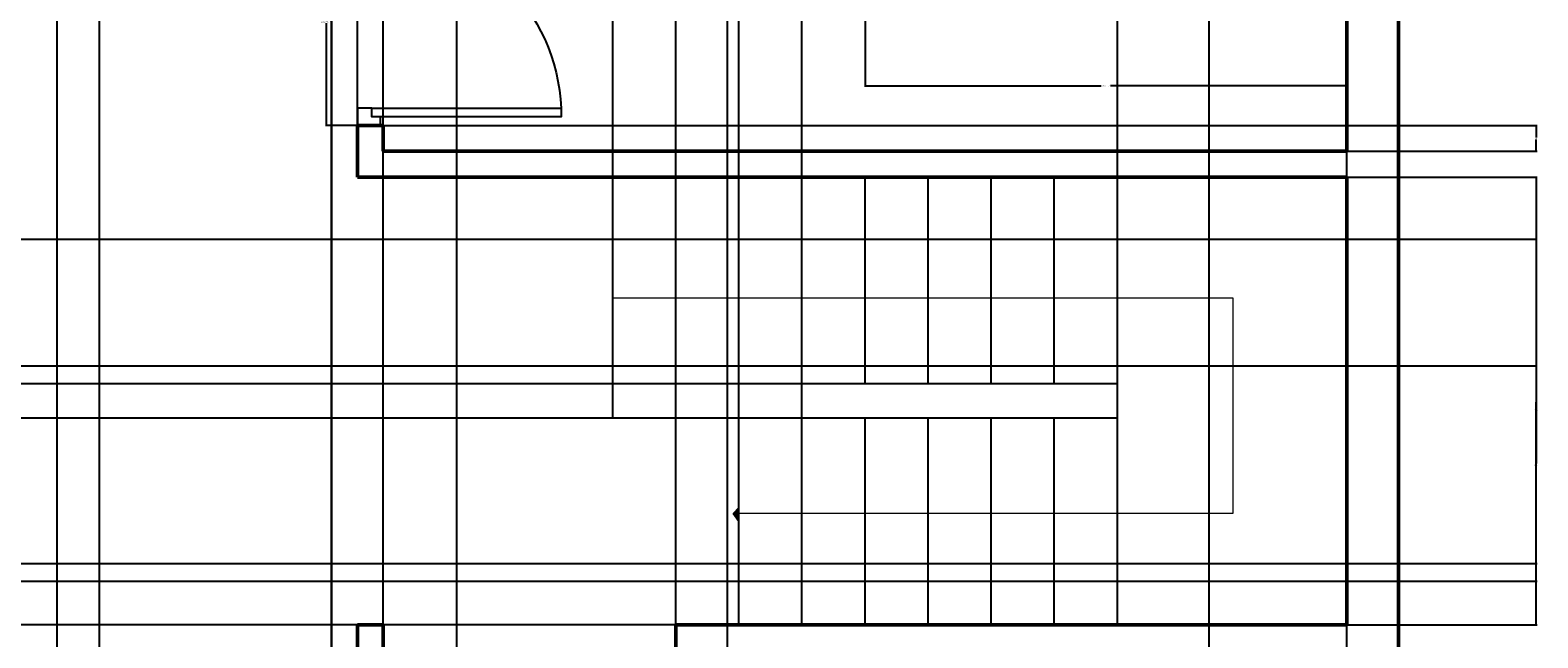
# Model space of a CAD drawing. Units: inches. Extents: x 2330 to 2739, y 947 to 1475.
# Tile 5 of 6: x 2476 to 2739, y 1185 to 1291. Entities that reach past the tile are written whole.
import ezdxf

# ---------------------------------------------------------------- set-up
doc = ezdxf.new("R2010")
doc.units = ezdxf.units.IN
for name, color, linetype, lineweight in [('A-ANNO-DIMS', 2, 'Continuous', 18), ('A-ANNO-SYMB', 7, 'Continuous', 18), ('door', 150, 'Continuous', 25), ('staircase', 51, 'Continuous', 25), ('wall', 7, 'Continuous', 50)]:
    doc.layers.add(name, color=color, linetype=linetype, lineweight=lineweight)
doc.styles.get("Standard").update_dxf_attribs({"font": 'arial.ttf'})
doc.dimstyles.get("Standard").update_dxf_attribs({"dimtxt": 0.18, "dimasz": 0.18, "dimexe": 0.18, "dimexo": 0.0625, "dimgap": 0.09, "dimtad": 0, "dimtih": 1, "dimtoh": 1, "dimdec": 4, "dimzin": 0, "dimdsep": 46, "dimtxsty": 'Standard', "dimcen": 0.09, "dimadec": 0, "dimazin": 0, "dimtfac": 1, "dimtdec": 4, "dimtofl": 0, "dimtmove": 0, "dimatfit": 3, "dimfxl": 1, "dimtolj": 1, "dimtzin": 0, "dimarcsym": 0})

# ---------------------------------------------------------------- blocks, each defined once
blk = doc.blocks.new('d1')
at = {"layer": 'door'}
blk.add_line((2897.27, 1313.4), (2933.27, 1313.4), dxfattribs=at)
blk.add_lwpolyline([(2898.77, 1315.9), (2900.27, 1315.9), (2900.27, 1348.9), (2898.77, 1348.9)], close=True, dxfattribs=at)
for points in [[(2900.27, 1313.4), (2897.27, 1313.4), (2897.27, 1317.4), (2898.77, 1317.4), (2898.77, 1315.9), (2900.27, 1315.9), (2900.27, 1313.4)], [(2930.27, 1313.4), (2933.27, 1313.4), (2933.27, 1317.4), (2931.77, 1317.4), (2931.77, 1315.9), (2930.27, 1315.9), (2930.27, 1313.4)]]:
    blk.add_lwpolyline(points, dxfattribs=at)
blk.add_arc((2898.77, 1315.9), 33.03, 2.6026, 87.3974, dxfattribs=at)
blk = doc.blocks.new('*D16')
at = {"layer": 'A-ANNO-DIMS', "color": 0, "lineweight": -2, "transparency": 16777216}
for p, q in [((2533.12, 1310.28), (2527.6, 1310.28)), ((2527.78, 1310.1), (2527.78, 1292.47)), ((2527.78, 1274.46), (2527.78, 1292.1)), ((2533.12, 1274.28), (2527.6, 1274.28))]:
    blk.add_line(p, q, dxfattribs=at)
at = {"layer": 'A-ANNO-DIMS', "color": 0, "transparency": 16777216}
for points in [[(2527.75, 1310.1), (2527.81, 1310.1), (2527.78, 1310.28)], [(2527.75, 1274.46), (2527.81, 1274.46), (2527.78, 1274.28)]]:
    blk.add_solid(points, dxfattribs=at)
at = {"layer": 'Defpoints', "color": 0, "transparency": 16777216}
for p in [(2527.78, 1310.28), (2533.18, 1310.28), (2533.18, 1274.28)]:
    blk.add_point(p, dxfattribs=at)
at = {"layer": 'A-ANNO-DIMS', "color": 0, "transparency": 16777216, "insert": (2527.78, 1292.28), "char_height": 0.18, "attachment_point": 5}
blk.add_mtext('\\A1;DOOR D1 36 TYP.', dxfattribs=at)
blk = doc.blocks.new('*D18')
at = {"layer": 'A-ANNO-DIMS', "color": 0, "lineweight": -2, "transparency": 16777216}
for p, q in [((2621.68, 1293.72), (2621.68, 1281)), ((2705.68, 1293.72), (2705.68, 1281)), ((2621.86, 1281.18), (2662.86, 1281.18)), ((2705.5, 1281.18), (2664.5, 1281.18))]:
    blk.add_line(p, q, dxfattribs=at)
at = {"layer": 'A-ANNO-DIMS', "color": 0, "transparency": 16777216}
for points in [[(2621.86, 1281.21), (2621.86, 1281.15), (2621.68, 1281.18)], [(2705.5, 1281.21), (2705.5, 1281.15), (2705.68, 1281.18)]]:
    blk.add_solid(points, dxfattribs=at)
at = {"layer": 'Defpoints', "color": 0, "transparency": 16777216}
for p in [(2621.68, 1293.78), (2705.68, 1293.78), (2705.68, 1281.18)]:
    blk.add_point(p, dxfattribs=at)
at = {"layer": 'A-ANNO-DIMS', "color": 0, "transparency": 16777216, "insert": (2663.68, 1281.18), "char_height": 0.18, "attachment_point": 5}
blk.add_mtext('\\A1;BED 84 TYP.', dxfattribs=at)
blk = doc.blocks.new('*D27')
at = {"layer": 'A-ANNO-DIMS', "color": 0, "lineweight": -2, "transparency": 16777216}
for p, q in [((2537.68, 980.34), (2537.68, 1475.46)), ((2537.86, 1475.28), (2567.46, 1475.28)), ((2597.5, 1475.28), (2567.9, 1475.28)), ((2597.68, 980.34), (2597.68, 1475.46))]:
    blk.add_line(p, q, dxfattribs=at)
at = {"layer": 'A-ANNO-DIMS', "color": 0, "transparency": 16777216}
for points in [[(2537.86, 1475.31), (2537.86, 1475.25), (2537.68, 1475.28)], [(2597.5, 1475.31), (2597.5, 1475.25), (2597.68, 1475.28)]]:
    blk.add_solid(points, dxfattribs=at)
at = {"layer": 'Defpoints', "color": 0, "transparency": 16777216}
for p in [(2597.68, 1475.28), (2537.68, 980.28), (2597.68, 980.28)]:
    blk.add_point(p, dxfattribs=at)
at = {"layer": 'A-ANNO-DIMS', "color": 0, "transparency": 16777216, "insert": (2567.68, 1475.28), "char_height": 0.18, "attachment_point": 5}
blk.add_mtext('\\A1;60', dxfattribs=at)
blk = doc.blocks.new('*D32')
at = {"layer": 'A-ANNO-DIMS', "color": 0, "lineweight": -2, "transparency": 16777216}
for p, q in [((2705.74, 1265.28), (2738.86, 1265.28)), ((2738.68, 1265.1), (2738.68, 1226.46)), ((2738.68, 1187.46), (2738.68, 1226.1)), ((2705.74, 1187.28), (2738.86, 1187.28))]:
    blk.add_line(p, q, dxfattribs=at)
at = {"layer": 'A-ANNO-DIMS', "color": 0, "transparency": 16777216}
for points in [[(2738.65, 1265.1), (2738.71, 1265.1), (2738.68, 1265.28)], [(2738.65, 1187.46), (2738.71, 1187.46), (2738.68, 1187.28)]]:
    blk.add_solid(points, dxfattribs=at)
at = {"layer": 'Defpoints', "color": 0, "transparency": 16777216}
for p in [(2705.68, 1265.28), (2738.68, 1265.28), (2705.68, 1187.28)]:
    blk.add_point(p, dxfattribs=at)
at = {"layer": 'A-ANNO-DIMS', "color": 0, "transparency": 16777216, "insert": (2738.68, 1226.28), "char_height": 0.18, "attachment_point": 5}
blk.add_mtext('\\A1;78', dxfattribs=at)
blk = doc.blocks.new('*D34')
at = {"layer": 'A-ANNO-DIMS', "color": 0, "lineweight": -2, "transparency": 16777216}
for p, q in [((2449.93, 1139.34), (2449.93, 1475.46)), ((2450.11, 1475.28), (2468.66, 1475.28)), ((2488, 1475.28), (2469.45, 1475.28)), ((2488.18, 1139.34), (2488.18, 1475.46))]:
    blk.add_line(p, q, dxfattribs=at)
at = {"layer": 'A-ANNO-DIMS', "color": 0, "transparency": 16777216}
for points in [[(2450.11, 1475.31), (2450.11, 1475.25), (2449.93, 1475.28)], [(2488, 1475.31), (2488, 1475.25), (2488.18, 1475.28)]]:
    blk.add_solid(points, dxfattribs=at)
at = {"layer": 'Defpoints', "color": 0, "transparency": 16777216}
for p in [(2488.18, 1475.28), (2449.93, 1139.28), (2488.18, 1139.28)]:
    blk.add_point(p, dxfattribs=at)
at = {"layer": 'A-ANNO-DIMS', "color": 0, "transparency": 16777216, "insert": (2469.05, 1475.28), "char_height": 0.18, "attachment_point": 5}
blk.add_mtext('\\A1;38.25', dxfattribs=at)
blk = doc.blocks.new('*D36')
at = {"layer": 'A-ANNO-DIMS', "color": 0, "lineweight": -2, "transparency": 16777216}
for p, q in [((2528.68, 1394.22), (2528.68, 947.1)), ((2550.43, 1394.22), (2550.43, 947.1)), ((2528.86, 947.28), (2539.16, 947.28)), ((2550.25, 947.28), (2539.95, 947.28))]:
    blk.add_line(p, q, dxfattribs=at)
at = {"layer": 'A-ANNO-DIMS', "color": 0, "transparency": 16777216}
for points in [[(2528.86, 947.31), (2528.86, 947.25), (2528.68, 947.28)], [(2550.25, 947.31), (2550.25, 947.25), (2550.43, 947.28)]]:
    blk.add_solid(points, dxfattribs=at)
at = {"layer": 'Defpoints', "color": 0, "transparency": 16777216}
for p in [(2528.68, 1394.28), (2550.43, 1394.28), (2550.43, 947.28)]:
    blk.add_point(p, dxfattribs=at)
at = {"layer": 'A-ANNO-DIMS', "color": 0, "transparency": 16777216, "insert": (2539.55, 947.28), "char_height": 0.18, "attachment_point": 5}
blk.add_mtext('\\A1;21.75', dxfattribs=at)
blk = doc.blocks.new('*D38')
at = {"layer": 'A-ANNO-DIMS', "color": 0, "lineweight": -2, "transparency": 16777216}
for p, q in [((2537.68, 1134.84), (2537.68, 1475.46)), ((2537.86, 1475.28), (2562.98, 1475.28)), ((2588.5, 1475.28), (2563.38, 1475.28)), ((2588.68, 1134.84), (2588.68, 1475.46))]:
    blk.add_line(p, q, dxfattribs=at)
at = {"layer": 'A-ANNO-DIMS', "color": 0, "transparency": 16777216}
for points in [[(2537.86, 1475.31), (2537.86, 1475.25), (2537.68, 1475.28)], [(2588.5, 1475.31), (2588.5, 1475.25), (2588.68, 1475.28)]]:
    blk.add_solid(points, dxfattribs=at)
at = {"layer": 'Defpoints', "color": 0, "transparency": 16777216}
for p in [(2588.68, 1475.28), (2537.68, 1134.78), (2588.68, 1134.78)]:
    blk.add_point(p, dxfattribs=at)
at = {"layer": 'A-ANNO-DIMS', "color": 0, "transparency": 16777216, "insert": (2563.18, 1475.28), "char_height": 0.18, "attachment_point": 5}
blk.add_mtext('\\A1;51', dxfattribs=at)
blk = doc.blocks.new('*D40')
at = {"layer": 'A-ANNO-DIMS', "color": 0, "lineweight": -2, "transparency": 16777216}
for p, q in [((2537.74, 1274.28), (2738.86, 1274.28)), ((2738.68, 1274.1), (2738.68, 1272.21)), ((2537.74, 1269.78), (2738.86, 1269.78)), ((2738.68, 1269.96), (2738.68, 1271.85))]:
    blk.add_line(p, q, dxfattribs=at)
at = {"layer": 'A-ANNO-DIMS', "color": 0, "transparency": 16777216}
for points in [[(2738.65, 1274.1), (2738.71, 1274.1), (2738.68, 1274.28)], [(2738.65, 1269.96), (2738.71, 1269.96), (2738.68, 1269.78)]]:
    blk.add_solid(points, dxfattribs=at)
at = {"layer": 'Defpoints', "color": 0, "transparency": 16777216}
for p in [(2537.68, 1274.28), (2738.68, 1274.28), (2537.68, 1269.78)]:
    blk.add_point(p, dxfattribs=at)
at = {"layer": 'A-ANNO-DIMS', "color": 0, "transparency": 16777216, "insert": (2738.68, 1272.03), "char_height": 0.18, "attachment_point": 5}
blk.add_mtext('\\A1;4.5', dxfattribs=at)
blk = doc.blocks.new('*D45')
at = {"layer": 'A-ANNO-DIMS', "color": 0, "lineweight": -2, "transparency": 16777216}
for p, q in [((2397.62, 1254.48), (2738.86, 1254.48)), ((2738.68, 1254.3), (2738.68, 1224.87)), ((2738.68, 1195.08), (2738.68, 1224.51)), ((2397.62, 1194.9), (2738.86, 1194.9))]:
    blk.add_line(p, q, dxfattribs=at)
at = {"layer": 'A-ANNO-DIMS', "color": 0, "transparency": 16777216}
for points in [[(2738.65, 1254.3), (2738.71, 1254.3), (2738.68, 1254.48)], [(2738.65, 1195.08), (2738.71, 1195.08), (2738.68, 1194.9)]]:
    blk.add_solid(points, dxfattribs=at)
at = {"layer": 'Defpoints', "color": 0, "transparency": 16777216}
for p in [(2397.55, 1254.48), (2397.55, 1194.9), (2738.68, 1194.9)]:
    blk.add_point(p, dxfattribs=at)
at = {"layer": 'A-ANNO-DIMS', "color": 0, "transparency": 16777216, "insert": (2738.68, 1224.69), "char_height": 0.18, "attachment_point": 5}
blk.add_mtext('\\A1;59.59', dxfattribs=at)
blk = doc.blocks.new('*D47')
at = {"layer": 'A-ANNO-DIMS', "color": 0, "lineweight": -2, "transparency": 16777216}
for p, q in [((2453.1, 1232.41), (2738.86, 1232.41)), ((2738.68, 1232.23), (2738.68, 1215.37)), ((2738.68, 1198.15), (2738.68, 1215.01)), ((2453.1, 1197.97), (2738.86, 1197.97))]:
    blk.add_line(p, q, dxfattribs=at)
at = {"layer": 'A-ANNO-DIMS', "color": 0, "transparency": 16777216}
for points in [[(2738.65, 1232.23), (2738.71, 1232.23), (2738.68, 1232.41)], [(2738.65, 1198.15), (2738.71, 1198.15), (2738.68, 1197.97)]]:
    blk.add_solid(points, dxfattribs=at)
at = {"layer": 'Defpoints', "color": 0, "transparency": 16777216}
for p in [(2453.04, 1232.41), (2453.04, 1197.97), (2738.68, 1197.97)]:
    blk.add_point(p, dxfattribs=at)
at = {"layer": 'A-ANNO-DIMS', "color": 0, "transparency": 16777216, "insert": (2738.68, 1215.19), "char_height": 0.18, "attachment_point": 5}
blk.add_mtext('\\A1;34.45', dxfattribs=at)
blk = doc.blocks.new('*D72')
at = {"layer": 'A-ANNO-DIMS', "color": 0, "lineweight": -2, "transparency": 16777216}
for p, q in [((2599.68, 1187.34), (2599.68, 1475.46)), ((2599.86, 1475.28), (2604.99, 1475.28)), ((2610.5, 1475.28), (2605.37, 1475.28)), ((2610.68, 1187.34), (2610.68, 1475.46))]:
    blk.add_line(p, q, dxfattribs=at)
at = {"layer": 'A-ANNO-DIMS', "color": 0, "transparency": 16777216}
for points in [[(2599.86, 1475.31), (2599.86, 1475.25), (2599.68, 1475.28)], [(2610.5, 1475.31), (2610.5, 1475.25), (2610.68, 1475.28)]]:
    blk.add_solid(points, dxfattribs=at)
at = {"layer": 'Defpoints', "color": 0, "transparency": 16777216}
for p in [(2610.68, 1475.28), (2599.68, 1187.28), (2610.68, 1187.28)]:
    blk.add_point(p, dxfattribs=at)
at = {"layer": 'A-ANNO-DIMS', "color": 0, "transparency": 16777216, "insert": (2605.18, 1475.28), "char_height": 0.18, "attachment_point": 5}
blk.add_mtext('\\A1;11', dxfattribs=at)
blk = doc.blocks.new('*D73')
at = {"layer": 'A-ANNO-DIMS', "color": 0, "lineweight": -2, "transparency": 16777216}
for p, q in [((2588.62, 1223.28), (2330.5, 1223.28)), ((2330.68, 1223.1), (2330.68, 1205.46)), ((2330.68, 1187.46), (2330.68, 1205.1)), ((2588.62, 1187.28), (2330.5, 1187.28))]:
    blk.add_line(p, q, dxfattribs=at)
at = {"layer": 'A-ANNO-DIMS', "color": 0, "transparency": 16777216}
for points in [[(2330.65, 1223.1), (2330.71, 1223.1), (2330.68, 1223.28)], [(2330.65, 1187.46), (2330.71, 1187.46), (2330.68, 1187.28)]]:
    blk.add_solid(points, dxfattribs=at)
at = {"layer": 'Defpoints', "color": 0, "transparency": 16777216}
for p in [(2330.68, 1223.28), (2588.68, 1223.28), (2588.68, 1187.28)]:
    blk.add_point(p, dxfattribs=at)
at = {"layer": 'A-ANNO-DIMS', "color": 0, "transparency": 16777216, "insert": (2330.68, 1205.28), "char_height": 0.18, "attachment_point": 5}
blk.add_mtext('\\A1;36', dxfattribs=at)
blk = doc.blocks.new('*D74')
at = {"layer": 'A-ANNO-DIMS', "color": 0, "lineweight": -2, "transparency": 16777216}
for p, q in [((2665.62, 1229.28), (2330.5, 1229.28)), ((2330.68, 1229.1), (2330.68, 1226.46)), ((2330.68, 1223.46), (2330.68, 1226.1)), ((2665.62, 1223.28), (2330.5, 1223.28))]:
    blk.add_line(p, q, dxfattribs=at)
at = {"layer": 'A-ANNO-DIMS', "color": 0, "transparency": 16777216}
for points in [[(2330.65, 1229.1), (2330.71, 1229.1), (2330.68, 1229.28)], [(2330.65, 1223.46), (2330.71, 1223.46), (2330.68, 1223.28)]]:
    blk.add_solid(points, dxfattribs=at)
at = {"layer": 'Defpoints', "color": 0, "transparency": 16777216}
for p in [(2330.68, 1229.28), (2665.68, 1229.28), (2665.68, 1223.28)]:
    blk.add_point(p, dxfattribs=at)
at = {"layer": 'A-ANNO-DIMS', "color": 0, "transparency": 16777216, "insert": (2330.68, 1226.28), "char_height": 0.18, "attachment_point": 5}
blk.add_mtext('\\A1;6', dxfattribs=at)
blk = doc.blocks.new('*D75')
at = {"layer": 'A-ANNO-DIMS', "color": 0, "lineweight": -2, "transparency": 16777216}
for p, q in [((2665.68, 1187.34), (2665.68, 1475.46)), ((2665.86, 1475.28), (2685.46, 1475.28)), ((2705.5, 1475.28), (2685.9, 1475.28)), ((2705.68, 1187.34), (2705.68, 1475.46))]:
    blk.add_line(p, q, dxfattribs=at)
at = {"layer": 'A-ANNO-DIMS', "color": 0, "transparency": 16777216}
for points in [[(2665.86, 1475.31), (2665.86, 1475.25), (2665.68, 1475.28)], [(2705.5, 1475.31), (2705.5, 1475.25), (2705.68, 1475.28)]]:
    blk.add_solid(points, dxfattribs=at)
at = {"layer": 'Defpoints', "color": 0, "transparency": 16777216}
for p in [(2705.68, 1475.28), (2665.68, 1187.28), (2705.68, 1187.28)]:
    blk.add_point(p, dxfattribs=at)
at = {"layer": 'A-ANNO-DIMS', "color": 0, "transparency": 16777216, "insert": (2685.68, 1475.28), "char_height": 0.18, "attachment_point": 5}
blk.add_mtext('\\A1;40', dxfattribs=at)
blk = doc.blocks.new('*D76')
at = {"layer": 'A-ANNO-DIMS', "color": 0, "lineweight": -2, "transparency": 16777216}
for p, q in [((2577.68, 1265.34), (2577.68, 1475.46)), ((2577.86, 1475.28), (2621.46, 1475.28)), ((2665.5, 1475.28), (2621.9, 1475.28)), ((2665.68, 1265.34), (2665.68, 1475.46))]:
    blk.add_line(p, q, dxfattribs=at)
at = {"layer": 'A-ANNO-DIMS', "color": 0, "transparency": 16777216}
for points in [[(2577.86, 1475.31), (2577.86, 1475.25), (2577.68, 1475.28)], [(2665.5, 1475.31), (2665.5, 1475.25), (2665.68, 1475.28)]]:
    blk.add_solid(points, dxfattribs=at)
at = {"layer": 'Defpoints', "color": 0, "transparency": 16777216}
for p in [(2665.68, 1475.28), (2577.68, 1265.28), (2665.68, 1265.28)]:
    blk.add_point(p, dxfattribs=at)
at = {"layer": 'A-ANNO-DIMS', "color": 0, "transparency": 16777216, "insert": (2621.68, 1475.28), "char_height": 0.18, "attachment_point": 5}
blk.add_mtext('\\A1;88', dxfattribs=at)
blk = doc.blocks.new('*D78')
at = {"layer": 'A-ANNO-DIMS', "color": 0, "lineweight": -2, "transparency": 16777216}
for p, q in [((2681.68, 1182.84), (2681.68, 1475.46)), ((2681.86, 1475.28), (2693.46, 1475.28)), ((2705.5, 1475.28), (2693.9, 1475.28)), ((2705.68, 1182.84), (2705.68, 1475.46))]:
    blk.add_line(p, q, dxfattribs=at)
at = {"layer": 'A-ANNO-DIMS', "color": 0, "transparency": 16777216}
for points in [[(2681.86, 1475.31), (2681.86, 1475.25), (2681.68, 1475.28)], [(2705.5, 1475.31), (2705.5, 1475.25), (2705.68, 1475.28)]]:
    blk.add_solid(points, dxfattribs=at)
at = {"layer": 'Defpoints', "color": 0, "transparency": 16777216}
for p in [(2705.68, 1475.28), (2681.68, 1182.78), (2705.68, 1182.78)]:
    blk.add_point(p, dxfattribs=at)
at = {"layer": 'A-ANNO-DIMS', "color": 0, "transparency": 16777216, "insert": (2693.68, 1475.28), "char_height": 0.18, "attachment_point": 5}
blk.add_mtext('\\A1;24', dxfattribs=at)
blk = doc.blocks.new('*D80')
at = {"layer": 'A-ANNO-DIMS', "color": 0, "lineweight": -2, "transparency": 16777216}
for p, q in [((2480.81, 1118.34), (2480.81, 1475.46)), ((2480.99, 1475.28), (2504.34, 1475.28)), ((2528.5, 1475.28), (2505.14, 1475.28)), ((2528.68, 1118.34), (2528.68, 1475.46))]:
    blk.add_line(p, q, dxfattribs=at)
at = {"layer": 'A-ANNO-DIMS', "color": 0, "transparency": 16777216}
for points in [[(2480.99, 1475.31), (2480.99, 1475.25), (2480.81, 1475.28)], [(2528.5, 1475.31), (2528.5, 1475.25), (2528.68, 1475.28)]]:
    blk.add_solid(points, dxfattribs=at)
at = {"layer": 'Defpoints', "color": 0, "transparency": 16777216}
for p in [(2528.68, 1475.28), (2480.81, 1118.28), (2528.68, 1118.28)]:
    blk.add_point(p, dxfattribs=at)
at = {"layer": 'A-ANNO-DIMS', "color": 0, "transparency": 16777216, "insert": (2504.74, 1475.28), "char_height": 0.18, "attachment_point": 5}
blk.add_mtext('\\A1;47.87', dxfattribs=at)

msp = doc.modelspace()

# ---------------------------------------------------------------- hatches: boundary and pattern name
at = {"layer": 'A-ANNO-SYMB'}
h = msp.add_hatch(color=256, dxfattribs=at)
h.dxf.hatch_style = 1
h.paths.add_polyline_path([(2599.6781, 1205.2823), (2598.6765, 1206.7023), (2599.6781, 1207.7402)])

# ---------------------------------------------------------------- linework, layer by layer
for p, q in [((2577.6781, 1244.2823), (2685.8293, 1244.2823)), ((2685.8293, 1244.2823), (2685.8293, 1206.7023)), ((2599.6781, 1207.7402), (2598.6765, 1206.7023)), ((2599.6781, 1205.2823), (2598.6765, 1206.7023)), ((2599.6781, 1207.7402), (2599.6781, 1205.2823)), ((2685.8293, 1206.7023), (2599.6781, 1206.7023))]:
    msp.add_line(p, q, dxfattribs=at)
at = {"layer": 'staircase'}
for p, q in [((2577.6781, 1223.2823), (2577.6781, 1265.2823)), ((2588.6781, 1229.2823), (2588.6781, 1265.2823)), ((2599.6781, 1229.2823), (2599.6781, 1265.2823)), ((2610.6781, 1229.2823), (2610.6781, 1265.2823)), ((2621.6781, 1229.2823), (2621.6781, 1265.2823)), ((2632.6781, 1229.2823), (2632.6781, 1265.2823)), ((2643.6781, 1229.2823), (2643.6781, 1265.2823)), ((2654.6781, 1229.2823), (2654.6781, 1265.2823)), ((2665.6781, 1187.2823), (2665.6781, 1265.2823)), ((2665.6781, 1229.2823), (2577.6781, 1229.2823)), ((2665.6781, 1223.2823), (2577.6781, 1223.2823)), ((2588.6781, 1187.2823), (2588.6781, 1223.2823)), ((2599.6781, 1187.2823), (2599.6781, 1223.2823)), ((2610.6781, 1187.2823), (2610.6781, 1223.2823)), ((2621.6781, 1187.2823), (2621.6781, 1223.2823)), ((2632.6781, 1187.2823), (2632.6781, 1223.2823)), ((2643.6781, 1187.2823), (2643.6781, 1223.2823)), ((2654.6781, 1187.2823), (2654.6781, 1223.2823))]:
    msp.add_line(p, q, dxfattribs=at)
at = {"layer": 'wall'}
for p, q in [((2714.6781, 971.2823), (2714.6781, 1451.2823)), ((2705.6781, 1269.7823), (2705.6781, 1389.7823)), ((2533.1781, 1265.2823), (2533.1781, 1274.2823)), ((2537.6781, 1274.2823), (2533.1781, 1274.2823)), ((2537.6781, 1269.7823), (2537.6781, 1274.2823)), ((2705.6781, 1269.7823), (2537.6781, 1269.7823)), ((2705.6781, 1265.2823), (2533.1781, 1265.2823)), ((2705.6781, 1187.2823), (2705.6781, 1265.2823)), ((2533.1781, 1139.2823), (2533.1781, 1187.2823)), ((2537.6781, 1187.2823), (2533.1781, 1187.2823)), ((2537.6781, 1134.7823), (2537.6781, 1187.2823)), ((2705.6781, 1187.2823), (2588.6781, 1187.2823)), ((2588.6781, 1178.2823), (2588.6781, 1187.2823))]:
    msp.add_line(p, q, dxfattribs=at)

# ---------------------------------------------------------------- block references
at = {"layer": 'door', "xscale": -1, "rotation": 270}
msp.add_blockref('d1', (1219.7792, -1622.9868), dxfattribs=at)

# ---------------------------------------------------------------- dimensions: what is measured, and where the dimension line sits
at = {"layer": 'A-ANNO-DIMS'}
for base, p1, p2, override, picture, middle in [((2488.1781, 1475.2843), (2449.9281, 1139.2823), (2488.1781, 1139.2823), {"dimdec": 2, "dimlfac": 1, "dimrnd": 0, "dimzin": 0, "dimdsep": 46, "dimlunit": 2}, '*D34', (2469.0531, 1475.2843)), ((2528.6781, 1475.2843), (2480.806, 1118.2823), (2528.6781, 1118.2823), {"dimdec": 2, "dimlfac": 1, "dimrnd": 0, "dimzin": 0, "dimdsep": 46, "dimlunit": 2}, '*D80', (2504.7421, 1475.2843)), ((2597.6781, 1475.2843), (2537.6781, 980.2823), (2597.6781, 980.2823), {"dimdec": 0, "dimlfac": 1, "dimrnd": 0, "dimzin": 0, "dimdsep": 46, "dimlunit": 2}, '*D27', (2567.6781, 1475.2843)), ((2588.6781, 1475.2843), (2537.6781, 1134.7823), (2588.6781, 1134.7823), {"dimdec": 0, "dimlfac": 1, "dimrnd": 0, "dimzin": 0, "dimdsep": 46, "dimlunit": 2}, '*D38', (2563.1781, 1475.2843)), ((2665.6781, 1475.2843), (2577.6781, 1265.2823), (2665.6781, 1265.2823), {"dimdec": 0, "dimlfac": 1, "dimrnd": 0, "dimzin": 0, "dimdsep": 46, "dimlunit": 2}, '*D76', (2621.6781, 1475.2843)), ((2610.6781, 1475.2843), (2599.6781, 1187.2823), (2610.6781, 1187.2823), {"dimdec": 0, "dimlfac": 1, "dimrnd": 0, "dimzin": 0, "dimdsep": 46, "dimlunit": 2}, '*D72', (2605.1781, 1475.2843)), ((2705.6781, 1475.2843), (2665.6781, 1187.2823), (2705.6781, 1187.2823), {"dimdec": 0, "dimlfac": 1, "dimrnd": 0, "dimzin": 0, "dimdsep": 46, "dimlunit": 2}, '*D75', (2685.6781, 1475.2843)), ((2705.6781, 1475.2843), (2681.6781, 1182.7823), (2705.6781, 1182.7823), {"dimdec": 0, "dimlfac": 1, "dimrnd": 0, "dimzin": 0, "dimdsep": 46, "dimlunit": 2}, '*D78', (2693.6781, 1475.2843)), ((2550.4281, 947.2803), (2528.6781, 1394.2823), (2550.4281, 1394.2823), {"dimdec": 2, "dimlfac": 1, "dimrnd": 0, "dimzin": 0, "dimdsep": 46, "dimlunit": 2}, '*D36', (2539.5531, 947.2803))]:
    dim = msp.add_linear_dim(base=base, p1=p1, p2=p2, dimstyle='Standard', override=override, dxfattribs=at)
    dim.commit()
    dim.dimension.update_dxf_attribs({"geometry": picture, "text_midpoint": middle})
dim = msp.add_linear_dim(base=(2527.7781, 1310.2823), p1=(2533.1781, 1274.2823), p2=(2533.1781, 1310.2823), angle=90, text='DOOR D1 <> TYP.', dimstyle='Standard', override={"dimdec": 0, "dimlfac": 1, "dimrnd": 0, "dimzin": 0, "dimdsep": 46, "dimlunit": 2}, dxfattribs=at)
dim.commit()
dim.dimension.update_dxf_attribs({"geometry": '*D16', "text_midpoint": (2527.7781, 1292.2823)})
dim = msp.add_linear_dim(base=(2705.6781, 1281.1823), p1=(2621.6781, 1293.7823), p2=(2705.6781, 1293.7823), text='BED <> TYP.', dimstyle='Standard', override={"dimdec": 0, "dimlfac": 1, "dimrnd": 0, "dimzin": 0, "dimdsep": 46, "dimlunit": 2}, dxfattribs=at)
dim.commit()
dim.dimension.update_dxf_attribs({"geometry": '*D18', "text_midpoint": (2663.6781, 1281.1823)})
for base, p1, p2, override, picture, middle in [((2738.6801, 1274.2823), (2537.6781, 1269.7823), (2537.6781, 1274.2823), {"dimdec": 1, "dimlfac": 1, "dimrnd": 0, "dimzin": 0, "dimdsep": 46, "dimlunit": 2}, '*D40', (2738.6801, 1272.0323)), ((2738.6801, 1265.2823), (2705.6781, 1187.2823), (2705.6781, 1265.2823), {"dimdec": 0, "dimlfac": 1, "dimrnd": 0, "dimzin": 0, "dimdsep": 46, "dimlunit": 2}, '*D32', (2738.6801, 1226.2823)), ((2738.6801, 1194.8972), (2397.5542, 1254.4842), (2397.5542, 1194.8972), {"dimdec": 2, "dimlfac": 1, "dimrnd": 0, "dimzin": 0, "dimdsep": 46, "dimlunit": 2}, '*D45', (2738.6801, 1224.6907)), ((2738.6801, 1197.968), (2453.0384, 1232.4146), (2453.0384, 1197.968), {"dimdec": 2, "dimlfac": 1, "dimrnd": 0, "dimzin": 0, "dimdsep": 46, "dimlunit": 2}, '*D47', (2738.6801, 1215.1913)), ((2330.6761, 1229.2823), (2665.6781, 1223.2823), (2665.6781, 1229.2823), {"dimdec": 0, "dimlfac": 1, "dimrnd": 0, "dimzin": 0, "dimdsep": 46, "dimlunit": 2}, '*D74', (2330.6761, 1226.2823)), ((2330.6761, 1223.2823), (2588.6781, 1187.2823), (2588.6781, 1223.2823), {"dimdec": 0, "dimlfac": 1, "dimrnd": 0, "dimzin": 0, "dimdsep": 46, "dimlunit": 2}, '*D73', (2330.6761, 1205.2823))]:
    dim = msp.add_linear_dim(base=base, p1=p1, p2=p2, angle=90, dimstyle='Standard', override=override, dxfattribs=at)
    dim.commit()
    dim.dimension.update_dxf_attribs({"geometry": picture, "text_midpoint": middle})

doc.saveas('drawing.dxf')
